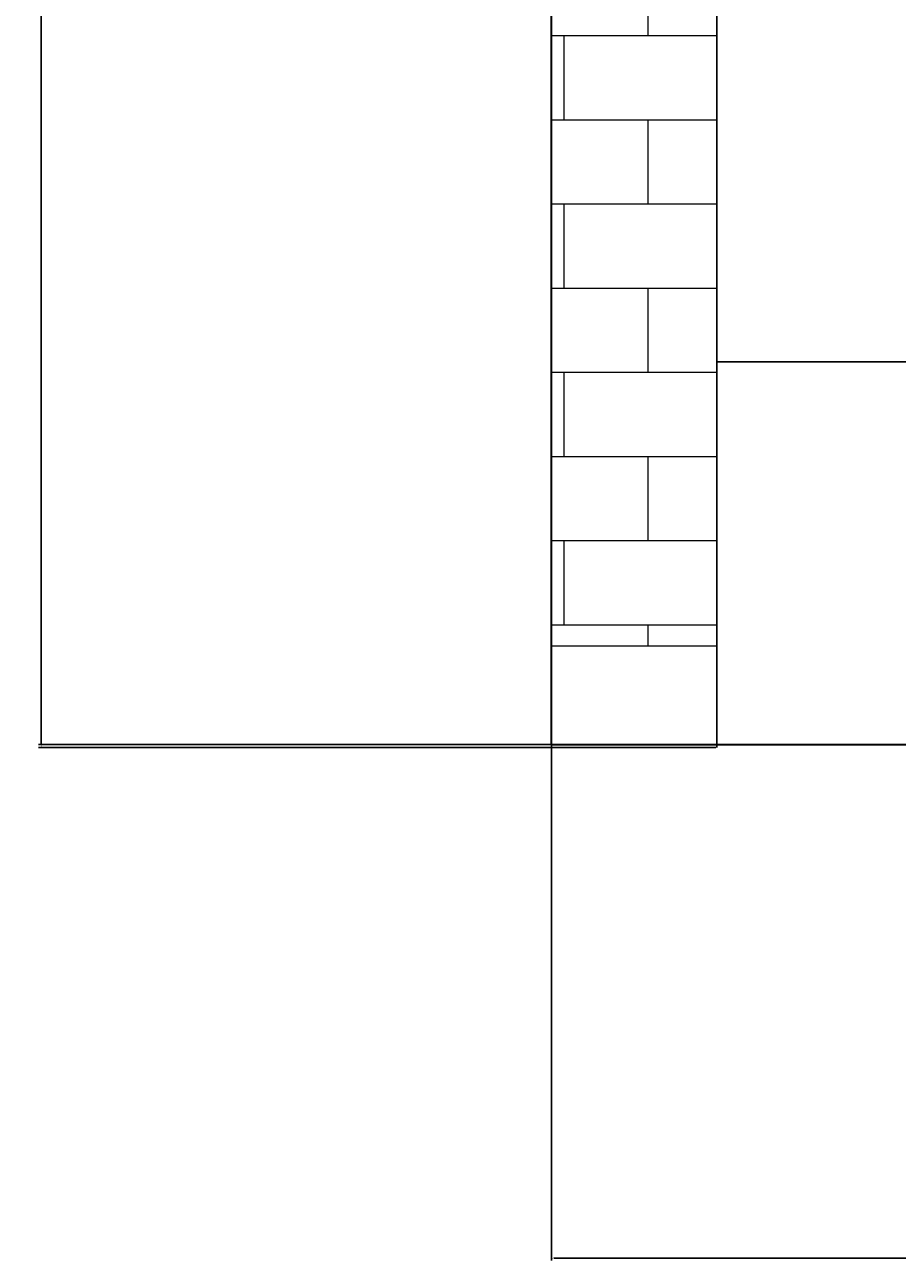
# Model space of a CAD drawing. Units: inches. Extents: x -26 to 776, y -22 to 650.
# Tile 1 of 62: x -26 to 36, y -22 to 67. Entities that reach past the tile are written whole.
import ezdxf

# ---------------------------------------------------------------- set-up
doc = ezdxf.new("R2010")
doc.units = ezdxf.units.IN
doc.header["$MEASUREMENT"] = 0
for name, color, linetype, lineweight in [('A-ANNO-DIMS', 2, 'Continuous', 18), ('A-DOOR', 3, 'Continuous', 25), ('A-WALL', 7, 'Continuous', 35), ('A-WALL-PATT', 8, 'Continuous', 13), ('A-WALL-TRIM', 7, 'Continuous', 18), ('C-TOPO', 7, 'Continuous', 35)]:
    doc.layers.add(name, color=color, linetype=linetype, lineweight=lineweight)
doc.styles.get("Standard").update_dxf_attribs({"font": 'arial.ttf'})
doc.dimstyles.get("Standard").update_dxf_attribs({"dimtxt": 0.5625, "dimasz": 0.18, "dimexe": 0.18, "dimexo": 0.0625, "dimgap": 0.09, "dimtad": 0, "dimtih": 1, "dimtoh": 1, "dimdec": 4, "dimzin": 0, "dimdsep": 46, "dimlunit": 4, "dimtxsty": 'Standard', "dimcen": 0.09, "dimadec": 0, "dimazin": 0, "dimtfac": 1, "dimtdec": 4, "dimtofl": 0, "dimtmove": 0, "dimatfit": 3, "dimfxl": 1, "dimtolj": 1, "dimtzin": 0, "dimarcsym": 0})

# ---------------------------------------------------------------- blocks, each defined once
blk = doc.blocks.new('*D13')
at = {"layer": 'A-ANNO-DIMS', "color": 0, "lineweight": -2, "transparency": 16777216}
for p, q in [((738.75, 50.786), (738.75, -21.315)), ((11.107, 15.42), (11.107, -21.315)), ((11.287, -21.135), (373.892, -21.135)), ((738.57, -21.135), (375.965, -21.135))]:
    blk.add_line(p, q, dxfattribs=at)
at = {"layer": 'A-ANNO-DIMS', "color": 0, "transparency": 16777216}
for points in [[(11.287, -21.105), (11.287, -21.165), (11.107, -21.135)], [(738.57, -21.105), (738.57, -21.165), (738.75, -21.135)]]:
    blk.add_solid(points, dxfattribs=at)
at = {"layer": 'Defpoints', "color": 0, "transparency": 16777216}
for p in [(738.75, 50.848), (11.107, 15.482), (738.75, -21.135)]:
    blk.add_point(p, dxfattribs=at)
at = {"layer": 'A-ANNO-DIMS', "color": 0, "transparency": 16777216, "insert": (374.929, -21.135), "char_height": 0.5625, "attachment_point": 5}
blk.add_mtext('\\A1;727.6', dxfattribs=at)
blk = doc.blocks.new('*D14')
at = {"layer": 'A-ANNO-DIMS', "color": 0, "lineweight": -2, "transparency": 16777216}
for p, q in [((191.616, 613.271), (-25.478, 613.271)), ((-25.298, 613.091), (-25.298, 314.754)), ((-25.298, 15.662), (-25.298, 314)), ((11.045, 15.482), (-25.478, 15.482))]:
    blk.add_line(p, q, dxfattribs=at)
at = {"layer": 'A-ANNO-DIMS', "color": 0, "transparency": 16777216}
for points in [[(-25.328, 613.091), (-25.268, 613.091), (-25.298, 613.271)], [(-25.328, 15.662), (-25.268, 15.662), (-25.298, 15.482)]]:
    blk.add_solid(points, dxfattribs=at)
at = {"layer": 'Defpoints', "color": 0, "transparency": 16777216}
for p in [(-25.298, 613.271), (191.678, 613.271), (11.107, 15.482)]:
    blk.add_point(p, dxfattribs=at)
at = {"layer": 'A-ANNO-DIMS', "color": 0, "transparency": 16777216, "insert": (-25.298, 314.377), "char_height": 0.5625, "attachment_point": 5}
blk.add_mtext('\\A1;597.8', dxfattribs=at)
blk = doc.blocks.new('*D22')
at = {"layer": 'A-ANNO-DIMS', "color": 0, "lineweight": -2, "transparency": 16777216}
for p, q in [((22.889, 15.333), (22.889, 649.856)), ((217.953, 15.545), (217.953, 649.856)), ((23.069, 649.676), (119.19, 649.676)), ((217.773, 649.676), (121.652, 649.676))]:
    blk.add_line(p, q, dxfattribs=at)
at = {"layer": 'A-ANNO-DIMS', "color": 0, "transparency": 16777216}
for points in [[(23.069, 649.706), (23.069, 649.646), (22.889, 649.676)], [(217.773, 649.706), (217.773, 649.646), (217.953, 649.676)]]:
    blk.add_solid(points, dxfattribs=at)
at = {"layer": 'Defpoints', "color": 0, "transparency": 16777216}
for p in [(217.953, 649.676), (22.889, 15.27), (217.953, 15.482)]:
    blk.add_point(p, dxfattribs=at)
at = {"layer": 'A-ANNO-DIMS', "color": 0, "transparency": 16777216, "insert": (120.421, 649.676), "char_height": 0.5625, "attachment_point": 5}
blk.add_mtext('\\A1;195.06', dxfattribs=at)
blk = doc.blocks.new('*D23')
at = {"layer": 'A-ANNO-DIMS', "color": 0, "lineweight": -2, "transparency": 16777216}
for p, q in [((22.827, 138.384), (-25.478, 138.384)), ((-25.298, 138.204), (-25.298, 77.205)), ((-25.298, 15.45), (-25.298, 76.45)), ((22.827, 15.27), (-25.478, 15.27))]:
    blk.add_line(p, q, dxfattribs=at)
at = {"layer": 'A-ANNO-DIMS', "color": 0, "transparency": 16777216}
for points in [[(-25.328, 138.204), (-25.268, 138.204), (-25.298, 138.384)], [(-25.328, 15.45), (-25.268, 15.45), (-25.298, 15.27)]]:
    blk.add_solid(points, dxfattribs=at)
at = {"layer": 'Defpoints', "color": 0, "transparency": 16777216}
for p in [(-25.298, 138.384), (22.889, 138.384), (22.889, 15.27)]:
    blk.add_point(p, dxfattribs=at)
at = {"layer": 'A-ANNO-DIMS', "color": 0, "transparency": 16777216, "insert": (-25.298, 76.827), "char_height": 0.5625, "attachment_point": 5}
blk.add_mtext('\\A1;123.11', dxfattribs=at)
blk = doc.blocks.new('*D24')
at = {"layer": 'A-ANNO-DIMS', "color": 0, "lineweight": -2, "transparency": 16777216}
for p, q in [((11.107, 15.545), (11.107, 649.856)), ((22.889, 15.333), (22.889, 649.856)), ((11.287, 649.676), (15.77, 649.676)), ((22.709, 649.676), (18.226, 649.676))]:
    blk.add_line(p, q, dxfattribs=at)
at = {"layer": 'A-ANNO-DIMS', "color": 0, "transparency": 16777216}
for points in [[(11.287, 649.706), (11.287, 649.646), (11.107, 649.676)], [(22.709, 649.706), (22.709, 649.646), (22.889, 649.676)]]:
    blk.add_solid(points, dxfattribs=at)
at = {"layer": 'Defpoints', "color": 0, "transparency": 16777216}
for p in [(22.889, 649.676), (11.107, 15.482), (22.889, 15.27)]:
    blk.add_point(p, dxfattribs=at)
at = {"layer": 'A-ANNO-DIMS', "color": 0, "transparency": 16777216, "insert": (16.998, 649.676), "char_height": 0.5625, "attachment_point": 5}
blk.add_mtext('\\A1;11.782', dxfattribs=at)
blk = doc.blocks.new('*D37')
at = {"layer": 'A-ANNO-DIMS', "color": 0, "lineweight": -2, "transparency": 16777216}
for p, q in [((231.362, 159.482), (-25.478, 159.482)), ((-25.298, 159.302), (-25.298, 87.855)), ((-25.298, 15.662), (-25.298, 87.11)), ((217.89, 15.482), (-25.478, 15.482))]:
    blk.add_line(p, q, dxfattribs=at)
at = {"layer": 'A-ANNO-DIMS', "color": 0, "transparency": 16777216}
for points in [[(-25.328, 159.302), (-25.268, 159.302), (-25.298, 159.482)], [(-25.328, 15.662), (-25.268, 15.662), (-25.298, 15.482)]]:
    blk.add_solid(points, dxfattribs=at)
at = {"layer": 'Defpoints', "color": 0, "transparency": 16777216}
for p in [(-25.298, 159.482), (231.425, 159.482), (217.953, 15.482)]:
    blk.add_point(p, dxfattribs=at)
at = {"layer": 'A-ANNO-DIMS', "color": 0, "transparency": 16777216, "insert": (-25.298, 87.482), "char_height": 0.5625, "attachment_point": 5}
blk.add_mtext('\\A1;144', dxfattribs=at)

msp = doc.modelspace()

# ---------------------------------------------------------------- hatches: boundary and pattern name
at = {"layer": 'A-WALL-PATT'}
h = msp.add_hatch(dxfattribs=at)
h.set_pattern_fill('AR-B816', color=256, scale=0.75)
h.paths.add_polyline_path([(82.134, 209.6413), (11.1074, 209.6413), (11.1074, 159.4824), (82.134, 159.4824)])
h.paths.add_polyline_path([(231.4249, 209.6413), (209.091, 209.6413), (209.091, 159.4824), (214.1056, 159.4824), (214.1056, 199.3298), (231.4249, 199.3298)])
h.paths.add_polyline_path([(231.4249, 159.4824), (11.1074, 159.4824), (11.1074, 22.5014), (22.8891, 22.5014), (22.8891, 147.0781), (217.9529, 147.0781), (217.9529, 20.7937), (231.4249, 20.7937)])
h.paths.add_polyline_path([(285.0179, 152.3087), (280.6173, 144.8359), (280.6173, 26.4239), (240.1654, 26.4239), (240.1654, 144.8359), (231.4249, 159.4824), (231.4249, 20.7937), (285.0179, 20.7937)])

# ---------------------------------------------------------------- linework, layer by layer
at = {"layer": 'A-DOOR'}
for p, q in [((22.8891, 15.2701), (22.8891, 147.0781)), ((22.8891, 42.7535), (217.9529, 42.7535))]:
    msp.add_line(p, q, dxfattribs=at)
at = {"layer": 'A-WALL'}
msp.add_line((11.1074, 15.4824), (11.1074, 159.4824), dxfattribs=at)
at = {"layer": 'A-WALL-TRIM'}
msp.add_line((11.1074, 22.5014), (22.8891, 22.5014), dxfattribs=at)
at = {"layer": 'C-TOPO'}
msp.add_line((11.1074, 15.4824), (92.2983, 15.4824), dxfattribs=at)

# ---------------------------------------------------------------- dimensions: what is measured, and where the dimension line sits
at = {"layer": 'A-ANNO-DIMS'}
for base, p1, p2, override, picture, middle in [((22.8891, 649.6763), (11.1074, 15.4824), (22.8891, 15.2701), {"dimdec": 3, "dimlfac": 1, "dimrnd": 0, "dimzin": 0, "dimdsep": 46, "dimlunit": 2}, '*D24', (16.9982, 649.6763)), ((217.9529, 649.6763), (22.8891, 15.2701), (217.9529, 15.4824), {"dimdec": 2, "dimlfac": 1, "dimrnd": 0, "dimzin": 0, "dimdsep": 46, "dimlunit": 2}, '*D22', (120.421, 649.6763)), ((738.7503, -21.1349), (11.1074, 15.4824), (738.7503, 50.8482), {"dimdec": 1, "dimlfac": 1, "dimrnd": 0, "dimzin": 0, "dimdsep": 46, "dimlunit": 2}, '*D13', (374.9289, -21.1349))]:
    dim = msp.add_linear_dim(base=base, p1=p1, p2=p2, dimstyle='Standard', override=override, dxfattribs=at)
    dim.commit()
    dim.dimension.update_dxf_attribs({"geometry": picture, "text_midpoint": middle})
for base, p1, p2, override, picture, middle in [((-25.2976, 613.2713), (11.1074, 15.4824), (191.6782, 613.2713), {"dimdec": 1, "dimlfac": 1, "dimrnd": 0, "dimzin": 0, "dimdsep": 46, "dimlunit": 2}, '*D14', (-25.2976, 314.3769)), ((-25.2976, 159.4824), (217.9529, 15.4824), (231.4249, 159.4824), {"dimdec": 0, "dimlfac": 1, "dimrnd": 0, "dimzin": 0, "dimdsep": 46, "dimlunit": 2}, '*D37', (-25.2976, 87.4824)), ((-25.2976, 138.3844), (22.8891, 15.2701), (22.8891, 138.3844), {"dimdec": 2, "dimlfac": 1, "dimrnd": 0, "dimzin": 0, "dimdsep": 46, "dimlunit": 2}, '*D23', (-25.2976, 76.8273))]:
    dim = msp.add_linear_dim(base=base, p1=p1, p2=p2, angle=90, dimstyle='Standard', override=override, dxfattribs=at)
    dim.commit()
    dim.dimension.update_dxf_attribs({"geometry": picture, "text_midpoint": middle})

doc.saveas('drawing.dxf')
